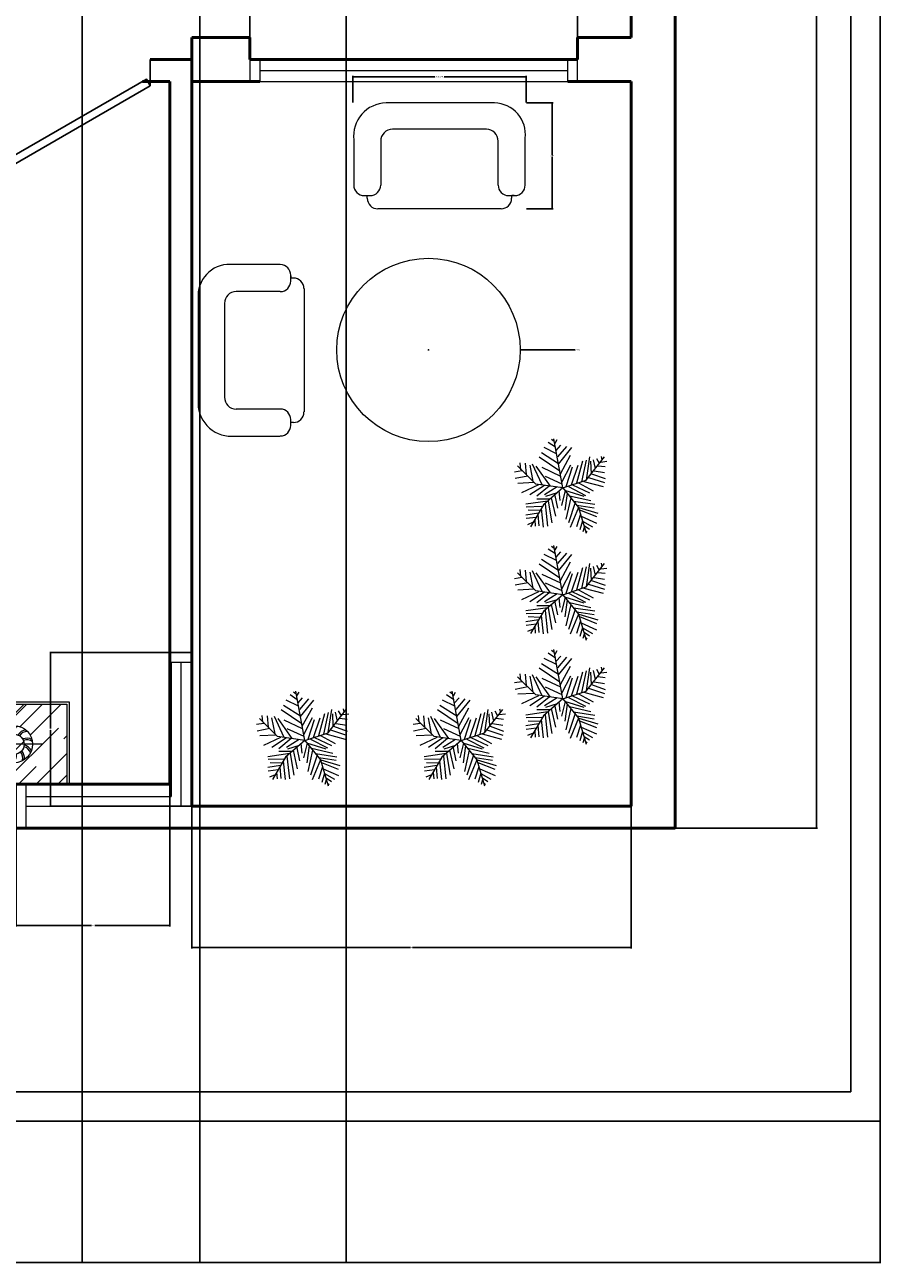
# Model space of a CAD drawing. Units: inches. Extents: x -28 to 483, y -584 to 51.
# Tile 3 of 6: x 270 to 445, y -584 to -330. Entities that reach past the tile are written whole.
import ezdxf

# ---------------------------------------------------------------- set-up
doc = ezdxf.new("R2010")
doc.units = ezdxf.units.IN
doc.header["$MEASUREMENT"] = 0
for name, color, linetype, lineweight in [('A-ANNO-DIMS', 2, 'Continuous', 18), ('A-DOOR', 4, 'Continuous', 25), ('A-FURN', 30, 'Continuous', 18), ('A-GLAZ', 5, 'Continuous', 18), ('A-WALL', 7, 'Continuous', 50), ('C-PROP', 7, 'Continuous', 25), ('tree', 3, 'Continuous', 13)]:
    doc.layers.add(name, color=color, linetype=linetype, lineweight=lineweight)
doc.styles.get("Standard").update_dxf_attribs({"font": 'arial.ttf'})
doc.dimstyles.get("Standard").update_dxf_attribs({"dimtxt": 0.18, "dimasz": 0.18, "dimexe": 0.18, "dimexo": 0.0625, "dimgap": 0.09, "dimtad": 0, "dimtih": 1, "dimtoh": 1, "dimdec": 4, "dimzin": 0, "dimdsep": 46, "dimtxsty": 'Standard', "dimcen": 0.09, "dimadec": 0, "dimazin": 0, "dimtfac": 1, "dimtdec": 4, "dimtofl": 0, "dimtmove": 0, "dimatfit": 3, "dimfxl": 1, "dimtolj": 1, "dimtzin": 0, "dimarcsym": 0})

# ---------------------------------------------------------------- blocks, each defined once
blk = doc.blocks.new('*U2')
for p, q in [((0, 0), (0, -6)), ((40, 0), (40, -6))]:
    blk.add_line(p, q)
blk.add_lwpolyline([(0, 0), (34.64, 20), (35.52, 18.48), (0.87, -1.52)], close=True)
blk.add_arc((0, 0), 40, 0, 30)
blk = doc.blocks.new('A$C64B41DC1')
for p, q in [((0, 2.5079), (2.9903, 2.5079)), ((0, 2.0879), (0, 2.5079)), ((0.012, 2.4618), (0.0581, 2.5079)), ((0.012, 2.3515), (0.1684, 2.5079)), ((0.012, 2.0999), (0.012, 2.5079)), ((0.0543, 2.2213), (0.3409, 2.5079)), ((0.1689, 2.4179), (0.2589, 2.5079)), ((0.3265, 2.386), (0.4484, 2.5079)), ((0.3699, 2.3332), (0.5445, 2.5079)), ((0.548, 2.5079), (0.548, 2.0999)), ((0.56, 2.5079), (0.56, 2.0879)), ((0.6301, 2.5079), (0.6301, 0.4779)), ((0.6401, 2.461), (0.6401, 2.5079)), ((0.6401, 2.5079), (2.344, 2.5079)), ((2.344, 2.5079), (2.3601, 2.5079)), ((2.344, 2.5079), (2.344, 2.461)), ((2.3601, 2.5079), (2.3601, 2.4761)), ((2.3601, 0.4779), (2.3601, 2.5079)), ((2.4303, 2.5079), (2.4303, 2.0879)), ((2.4423, 2.5079), (2.4423, 2.0999)), ((2.4423, 2.3333), (2.6169, 2.5079)), ((2.4423, 2.2145), (2.7357, 2.5079)), ((2.4423, 2.404), (2.5354, 2.4971)), ((2.705, 2.398), (2.8149, 2.5079)), ((2.7691, 2.3772), (2.8998, 2.5079)), ((2.7819, 2.3646), (2.9252, 2.5079)), ((2.9783, 2.0999), (2.9783, 2.5079)), ((2.9903, 2.0879), (2.9903, 2.5079)), ((0.2157, 2.0999), (0.548, 2.4322)), ((0.2299, 2.0999), (0.548, 2.418)), ((0.2804, 2.1597), (0.2804, 2.4481)), ((2.344, 2.461), (0.6401, 2.461)), ((0.6601, 2.4461), (1.4951, 2.4461)), ((0.6601, 2.4461), (0.6601, 0.5579)), ((1.4951, 2.4461), (0.6697, 2.4461)), ((2.3301, 2.4461), (1.4951, 2.4461)), ((2.3301, 0.5579), (2.3301, 2.4461)), ((2.7099, 2.1597), (2.7099, 2.4481)), ((0.2311, 2.2906), (0.2937, 2.3532)), ((2.6674, 2.2756), (2.7382, 2.3464)), ((2.7914, 2.1846), (2.9783, 2.3715)), ((0.012, 2.261), (0.0275, 2.2765)), ((0.1362, 2.3039), (0.4246, 2.3039)), ((0.2905, 2.2539), (0.3304, 2.2938)), ((0.3405, 2.3039), (0.3605, 2.3238)), ((2.8541, 2.3039), (2.5657, 2.3039)), ((2.5849, 2.2779), (2.6158, 2.3088)), ((2.6158, 2.3088), (2.6313, 2.3243)), ((2.7249, 2.3076), (2.7512, 2.3339)), ((2.7746, 2.0999), (2.9783, 2.3036)), ((2.9144, 2.2312), (2.9783, 2.2951)), ((0.0404, 2.0999), (0.1982, 2.2578)), ((0.1365, 2.0999), (0.251, 2.2144)), ((0.4194, 2.0999), (0.548, 2.2285)), ((2.4423, 2.1353), (2.5382, 2.2312)), ((2.4918, 2.0999), (2.6366, 2.2447)), ((0.4986, 2.0999), (0.548, 2.1493)), ((2.7831, 2.0999), (2.8678, 2.1846)), ((2.8962, 2.0999), (2.9783, 2.182)), ((0.56, 2.0879), (0, 2.0879)), ((0.548, 2.0999), (0.012, 2.0999)), ((0.5127, 2.0999), (0.548, 2.1352)), ((2.4303, 2.0879), (2.9903, 2.0879)), ((2.4423, 2.0999), (2.9783, 2.0999)), ((2.5172, 2.0999), (2.5269, 2.1096)), ((0.9415, 1.9902), (0.9415, 1.3975)), ((0.9715, 1.9906), (0.9715, 1.4076)), ((1.0015, 1.991), (1.0015, 1.4177)), ((1.0315, 1.9916), (1.0315, 1.4279)), ((2.3349, 1.8678), (0.6613, 1.3029)), ((0.8956, 1.1191), (2.3349, 1.8678)), ((1.6636, 1.6412), (0.6601, 1.6412)), ((1.5748, 1.6112), (0.6601, 1.6112)), ((2.3665, 1.295), (2.3665, 1.3839)), ((2.377, 1.295), (2.3822, 1.3891)), ((2.4032, 1.295), (2.4032, 1.3839)), ((2.4346, 1.295), (2.4346, 1.3839)), ((2.4451, 1.295), (2.4503, 1.3891)), ((2.4774, 1.2957), (2.4774, 1.3837)), ((2.5, 1.295), (2.5, 1.3839)), ((2.5105, 1.295), (2.5157, 1.3891)), ((2.5367, 1.295), (2.5367, 1.3839)), ((2.5471, 1.295), (2.5524, 1.3891)), ((2.5681, 1.295), (2.5681, 1.3839)), ((2.5918, 1.295), (2.5918, 1.3839)), ((2.6346, 1.2957), (2.6346, 1.3837)), ((2.6362, 1.2957), (2.6467, 1.3839)), ((2.6729, 1.295), (2.6624, 1.3839)), ((2.6938, 1.295), (2.6938, 1.3839)), ((2.7043, 1.295), (2.7095, 1.3891)), ((2.7127, 1.2957), (2.7232, 1.3839)), ((2.7253, 1.295), (2.7253, 1.3839)), ((2.7494, 1.295), (2.7389, 1.3839)), ((2.7718, 1.295), (2.7718, 1.3839)), ((2.7959, 1.295), (2.7854, 1.3839)), ((2.8146, 1.2957), (2.8146, 1.3837)), ((2.8146, 1.2957), (2.8146, 1.3837)), ((2.8282, 1.295), (2.8282, 1.3839)), ((2.8282, 1.295), (2.8282, 1.3839)), ((2.8523, 1.295), (2.8418, 1.3839)), ((2.8523, 1.295), (2.8418, 1.3839)), ((2.8653, 1.2966), (2.8688, 1.3861)), ((2.8711, 1.2957), (2.8711, 1.3837)), ((2.8711, 1.2957), (2.8875, 1.3822)), ((2.8713, 1.2927), (2.954, 1.3315)), ((2.8765, 1.2958), (2.9132, 1.3758)), ((2.8893, 1.3011), (2.9394, 1.3636)), ((2.3601, 1.2873), (2.8639, 1.2873)), ((2.8639, 1.2873), (2.8639, 0.1018)), ((2.8716, 1.2565), (2.9605, 1.2669)), ((2.8717, 1.2884), (2.9588, 1.3058)), ((2.8744, 1.2817), (2.9603, 1.2869)), ((2.3601, 1.2233), (2.7999, 1.2233)), ((2.7999, 1.2233), (2.7999, 0.1658)), ((2.8716, 1.2212), (2.9605, 1.2212)), ((2.8716, 1.1947), (2.9605, 1.2052)), ((2.8723, 1.2489), (2.9603, 1.2489)), ((2.3601, 1.1913), (2.7679, 1.1912)), ((2.7679, 1.1912), (2.7679, 0.1978)), ((2.8716, 1.181), (2.9605, 1.1705)), ((2.8716, 1.1595), (2.9605, 1.1595)), ((2.8716, 1.133), (2.9605, 1.1435)), ((2.8723, 1.1872), (2.9603, 1.1872)), ((2.8716, 1.1193), (2.9605, 1.1088)), ((2.8716, 1.1035), (2.9605, 1.093)), ((2.8716, 1.0965), (2.9605, 1.0965)), ((2.8716, 1.086), (2.9657, 1.0913)), ((2.8716, 1.0756), (2.9605, 1.0756)), ((2.8723, 1.1255), (2.9603, 1.1255)), ((2.8723, 1.0858), (2.9605, 1.0753)), ((2.8716, 1.0491), (2.9605, 1.0596)), ((2.8716, 1.0354), (2.9605, 1.0249)), ((2.8723, 1.0416), (2.9603, 1.0416)), ((2.8723, 0.9987), (2.9605, 1.0092)), ((2.8723, 0.985), (2.9605, 0.9745)), ((2.8723, 0.9735), (2.9603, 0.9735)), ((2.8716, 0.9346), (2.9605, 0.9241)), ((2.8723, 0.9408), (2.9603, 0.9408)), ((2.8723, 0.8979), (2.9605, 0.9084)), ((2.8723, 0.8726), (2.9603, 0.8726)), ((2.8723, 0.8505), (2.9603, 0.8505)), ((2.8716, 0.7885), (2.9605, 0.799)), ((2.8716, 0.7818), (2.9657, 0.787)), ((2.8716, 0.7503), (2.9657, 0.7556)), ((2.8716, 0.7204), (2.9605, 0.7309)), ((2.8716, 0.6995), (2.9605, 0.6995)), ((2.8723, 0.7571), (2.9605, 0.7466)), ((2.8716, 0.689), (2.9657, 0.6838)), ((2.8716, 0.6576), (2.9657, 0.6523)), ((2.8716, 0.6471), (2.9605, 0.6471)), ((2.8716, 0.5903), (2.9605, 0.6007)), ((0.7101, 0.5079), (2.2801, 0.5079)), ((2.882, 0.5582), (2.9657, 0.5536)), ((2.8909, 0.5263), (2.9657, 0.5222)), ((2.8928, 0.5169), (2.9605, 0.5169)), ((0.6301, 0.4779), (2.3601, 0.4779)), ((1.2465, 0.4625), (1.1576, 0.452)), ((1.2542, 0.1018), (1.2542, 0.4779)), ((1.3182, 0.1658), (1.3182, 0.4779)), ((1.3502, 0.1978), (1.3502, 0.4779)), ((2.8716, 0.4877), (2.9603, 0.4877)), ((2.8716, 0.4625), (2.9605, 0.452)), ((1.2465, 0.3746), (1.1576, 0.3851)), ((1.2465, 0.4365), (1.1577, 0.4365)), ((2.8716, 0.4365), (2.9603, 0.4365)), ((2.8716, 0.3746), (2.9605, 0.3851)), ((1.2465, 0.3684), (1.1577, 0.3684)), ((1.2285, 0.3357), (1.1577, 0.3357)), ((2.8716, 0.3684), (2.9603, 0.3684)), ((2.8896, 0.3357), (2.9603, 0.3357)), ((1.2355, 0.3092), (1.1576, 0.3)), ((1.2457, 0.2676), (1.1577, 0.2676)), ((2.8723, 0.2676), (2.9603, 0.2676)), ((2.8826, 0.3092), (2.9605, 0.3)), ((1.2457, 0.2423), (1.1576, 0.2319)), ((1.2465, 0.2057), (1.1576, 0.2161)), ((2.7679, 0.1978), (1.3502, 0.1978)), ((2.8716, 0.2057), (2.9605, 0.2161)), ((2.8723, 0.2423), (2.9605, 0.2319)), ((1.2465, 0.1742), (1.1524, 0.169)), ((1.2465, 0.1428), (1.1524, 0.1376)), ((1.2465, 0.1334), (1.1524, 0.1281)), ((1.2465, 0.1847), (1.1576, 0.1847)), ((1.2465, 0.1323), (1.1576, 0.1323)), ((1.2465, 0.1323), (1.1576, 0.1323)), ((2.7999, 0.1658), (1.3182, 0.1658)), ((2.8716, 0.1847), (2.9605, 0.1847)), ((2.8716, 0.1742), (2.9657, 0.169)), ((2.8716, 0.1428), (2.9657, 0.1376)), ((2.8716, 0.1334), (2.9657, 0.1281)), ((2.8716, 0.1323), (2.9605, 0.1323)), ((1.2465, 0.1), (1.1576, 0.1105)), ((1.2465, 0.1229), (1.1588, 0.1168)), ((1.2464, 0.1007), (1.1592, 0.0833)), ((1.2468, 0.0964), (1.1641, 0.0576)), ((1.2288, 0.088), (1.1787, 0.0255)), ((1.2415, 0.0933), (1.2049, 0.0133)), ((1.247, 0.0934), (1.2306, 0.0069)), ((1.2527, 0.0925), (1.2493, 0.003)), ((2.8639, 0.1018), (1.2542, 0.1018)), ((1.2658, 0.0941), (1.2762, 0.0052)), ((1.2899, 0.0941), (1.2899, 0.0052)), ((1.2999, 0.0941), (1.3051, 0)), ((1.3313, 0.0941), (1.3365, 0)), ((1.3523, 0.0941), (1.3575, 0)), ((1.3804, 0.0941), (1.3699, 0.0052)), ((1.4119, 0.0934), (1.4223, 0.0052)), ((1.4485, 0.0941), (1.438, 0.0052)), ((1.48, 0.0941), (1.4852, 0)), ((1.5114, 0.0941), (1.5166, 0)), ((1.5323, 0.0941), (1.5376, 0)), ((1.5638, 0.0941), (1.5638, 0.0105)), ((1.6021, 0.0941), (1.6021, 0.0052)), ((1.6336, 0.0941), (1.6336, 0.0052)), ((1.6702, 0.0941), (1.6702, 0.0052)), ((1.7017, 0.0941), (1.7017, 0.0052)), ((1.7122, 0.0941), (1.7174, 0)), ((1.7445, 0.0934), (1.7445, 0.0054)), ((1.7698, 0.0934), (1.7803, 0.0052)), ((1.8065, 0.0941), (1.796, 0.0052)), ((1.8274, 0.0941), (1.8274, 0.0052)), ((1.8379, 0.0941), (1.8431, 0)), ((1.8746, 0.0941), (1.8798, 0)), ((1.8955, 0.0941), (1.8955, 0.0052)), ((1.906, 0.0941), (1.9113, 0)), ((1.9384, 0.0934), (1.9384, 0.0054)), ((1.9609, 0.0941), (1.9609, 0.0052)), ((1.9636, 0.0934), (1.9741, 0.0052)), ((1.9714, 0.0941), (1.9766, 0)), ((1.9976, 0.0941), (1.9976, 0.0052)), ((2.0081, 0.0941), (2.0133, 0)), ((2.029, 0.0941), (2.029, 0.0052)), ((2.0395, 0.0941), (2.0447, 0)), ((2.0797, 0.0941), (2.0797, 0.0052)), ((2.0902, 0.0941), (2.0954, 0)), ((2.1216, 0.0941), (2.1269, 0)), ((2.1412, 0.0941), (2.1412, 0.0052)), ((2.1517, 0.0941), (2.1569, 0)), ((2.1831, 0.0941), (2.1884, 0)), ((2.2093, 0.0941), (2.2093, 0.0052)), ((2.2198, 0.0941), (2.225, 0)), ((2.2512, 0.0941), (2.2565, 0)), ((2.2603, 0.0934), (2.2707, 0.0052)), ((2.2969, 0.0941), (2.2864, 0.0052)), ((2.3089, 0.0934), (2.3193, 0.0052)), ((2.3455, 0.0941), (2.3351, 0.0052)), ((2.3665, 0.0941), (2.3665, 0.0052)), ((2.377, 0.0941), (2.3822, 0)), ((2.4032, 0.0941), (2.4032, 0.0052)), ((2.4346, 0.0941), (2.4346, 0.0052)), ((2.4451, 0.0941), (2.4503, 0)), ((2.4774, 0.0934), (2.4774, 0.0054)), ((2.5, 0.0941), (2.5, 0.0052)), ((2.5105, 0.0941), (2.5157, 0)), ((2.5367, 0.0941), (2.5367, 0.0052)), ((2.5471, 0.0941), (2.5524, 0)), ((2.5681, 0.0941), (2.5681, 0.0052)), ((2.5918, 0.0941), (2.5918, 0.0052)), ((2.6346, 0.0934), (2.6346, 0.0054)), ((2.6362, 0.0934), (2.6467, 0.0052)), ((2.6729, 0.0941), (2.6624, 0.0052)), ((2.6938, 0.0941), (2.6938, 0.0052)), ((2.7043, 0.0941), (2.7095, 0)), ((2.7127, 0.0934), (2.7232, 0.0052)), ((2.7253, 0.0941), (2.7253, 0.0052)), ((2.7494, 0.0941), (2.7389, 0.0052)), ((2.7718, 0.0941), (2.7718, 0.0052)), ((2.7959, 0.0941), (2.7854, 0.0052)), ((2.8146, 0.0934), (2.8146, 0.0054)), ((2.8282, 0.0941), (2.8282, 0.0052)), ((2.8523, 0.0941), (2.8418, 0.0052)), ((2.8653, 0.0925), (2.8688, 0.003)), ((2.8711, 0.0934), (2.8875, 0.0069)), ((2.8713, 0.0964), (2.954, 0.0576)), ((2.8716, 0.1229), (2.9593, 0.1168)), ((2.8717, 0.1007), (2.9588, 0.0833)), ((2.8744, 0.1074), (2.9603, 0.1022)), ((2.8765, 0.0933), (2.9132, 0.0133)), ((2.8893, 0.088), (2.9394, 0.0255))]:
    blk.add_line(p, q)
at = {"ltscale": 10}
for p, q in [((1.4859, 1.5812), (0.6601, 1.5812)), ((1.397, 1.5512), (0.6601, 1.5512))]:
    blk.add_line(p, q, dxfattribs=at)
for centre, radius in [((0.2804, 2.3039), 0.0942), ((0.2804, 2.3039), 0.051), ((2.7099, 2.3039), 0.0942), ((2.7099, 2.3039), 0.051)]:
    blk.add_circle(centre, radius)
for centre, radius, start, end in [((0.6601, 2.4761), 0.03, 180, 270), ((2.3301, 2.4761), 0.03, 270, 0), ((0.2417, 2.3614), 0.0462, 196.30017, 256.53802), ((0.2887, 2.3745), 0.0605, 172.17003, 218.48975), ((0.2828, 2.3731), 0.0462, 160.30017, 220.53802), ((0.3286, 2.3561), 0.0605, 136.17003, 182.48975), ((0.3231, 2.3585), 0.0462, 124.30017, 184.53802), ((0.3501, 2.3178), 0.0605, 100.17003, 146.48975), ((0.347, 2.323), 0.0462, 88.30017, 148.53802), ((1.0526, 2.3302), 0.3085, 175.30484, 198.69419), ((-0.8702, 2.0941), 1.6364, 4.80985, 9.18918), ((0.8579, 2.6278), 0.2948, 247.51785, 264.26696), ((0.728, 2.111), 0.245, 40.4189, 85.9871), ((1.0164, 5.7096), 3.3803, 266.81337, 276.16021), ((1.3963, 2.1044), 0.245, 94.0129, 139.5811), ((1.1858, 2.3288), 0.1943, 306.5711, 5.88998), ((1.5348, 2.2652), 0.1767, 151.77364, 201.69827), ((1.6986, 2.3355), 0.1943, 174.11002, 233.4289), ((1.1481, 2.2311), 0.3783, 353.49469, 19.18669), ((1.6871, 3.192), 0.8561, 257.74383, 273.62843), ((1.4882, 2.111), 0.245, 40.4189, 85.9871), ((1.8674, 1.9709), 0.3878, 68.20259, 108.9817), ((2.1269, 2.1044), 0.245, 94.0129, 139.5811), ((2.0342, 2.4856), 0.1563, 261.59582, 298.90918), ((1.9165, 2.3288), 0.1943, 333.73715, 5.88998), ((2.6058, 2.2028), 0.517, 163.60457, 172.3273), ((2.6433, 2.323), 0.0462, 31.46198, 91.69983), ((2.6402, 2.3178), 0.0605, 33.51025, 79.82997), ((2.6672, 2.3585), 0.0462, 355.46198, 55.69983), ((2.6617, 2.3561), 0.0605, 357.51025, 43.82997), ((2.7075, 2.3731), 0.0462, 319.46198, 19.69983), ((2.7016, 2.3745), 0.0605, 321.51025, 7.82997), ((2.7486, 2.3614), 0.0462, 283.46198, 343.69983), ((0.2153, 2.3276), 0.0462, 232.30017, 292.53802), ((0.2158, 2.3336), 0.0605, 244.17003, 290.48975), ((0.2457, 2.3659), 0.0605, 208.17003, 254.48975), ((0.3449, 2.2742), 0.0605, 64.17003, 110.48975), ((0.3455, 2.2802), 0.0462, 52.30017, 112.53802), ((0.3191, 2.2464), 0.0462, 16.30017, 76.53802), ((0.3151, 2.2419), 0.0605, 28.17003, 74.48975), ((2.6448, 2.2802), 0.0462, 67.46198, 127.69983), ((2.6454, 2.2742), 0.0605, 69.51025, 115.82997), ((2.6752, 2.2419), 0.0605, 105.51025, 151.82997), ((2.6712, 2.2464), 0.0462, 103.46198, 163.69983), ((2.7744, 2.3336), 0.0605, 249.51025, 295.82997), ((2.775, 2.3276), 0.0462, 247.46198, 307.69983), ((2.7446, 2.3659), 0.0605, 285.51025, 331.82997), ((0.2138, 2.2848), 0.0462, 268.30017, 328.53802), ((0.2107, 2.29), 0.0605, 280.17003, 326.48975), ((0.2377, 2.2493), 0.0462, 304.30017, 4.53802), ((0.2322, 2.2517), 0.0605, 316.17003, 2.48975), ((0.2779, 2.2347), 0.0462, 340.30017, 40.53802), ((0.272, 2.2333), 0.0605, 352.17003, 38.48975), ((0.7274, 2.2013), 0.0446, 314.4736, 42.17134), ((-1.6008, 2.277), 2.3618, 357.39054, 358.88764), ((1.9165, 2.3288), 0.1943, 320.94042, 333.73715), ((2.1347, 2.2313), 0.0459, 165.35061, 223.26844), ((2.7182, 2.2333), 0.0605, 141.51025, 187.82997), ((2.7123, 2.2347), 0.0462, 139.46198, 199.69983), ((2.7581, 2.2517), 0.0605, 177.51025, 223.82997), ((2.7526, 2.2493), 0.0462, 175.46198, 235.69983), ((2.7796, 2.29), 0.0605, 213.51025, 259.82997), ((2.7765, 2.2848), 0.0462, 211.46198, 271.69983), ((0.2688, 2.0945), 0.4956, 344.0243, 8.70709), ((1.204, 2.1778), 0.1681, 337.01697, 7.53676), ((1.5671, 2.1546), 0.0547, 142.08329, 220.902), ((1.9346, 2.1778), 0.1681, 337.01697, 7.53676), ((0.9385, 1.978), 0.1943, 126.5711, 185.88998), ((1.1858, 1.9714), 0.1943, 4.31813, 53.4289), ((1.5415, 2.0969), 0.1834, 175.22328, 196.23004), ((1.7059, 1.9714), 0.204, 127.11975, 175.09005), ((1.1965, 2.0983), 0.3299, 343.79543, 3.55541), ((1.9394, 1.991), 0.1651, 351.26213, 55.75721), ((2.4617, 2.0719), 0.3745, 173.82958, 196.4356), ((1.2687, 1.9248), 0.1223, 33.62799, 86.47438), ((1.7676, 1.0629), 0.9631, 69.65065, 105.96307), ((2.2748, 2.5795), 0.6373, 238.34989, 254.31375), ((0.7417, 2.0149), 0.057, 273.47085, 328.54118), ((0.728, 2.2025), 0.245, 274.0129, 278.34166), ((0.7246, 18.8439), 16.8552, 270.17399, 272.05214), ((1.3401, 1.9404), 0.0603, 49.09906, 101.37023), ((2.0911, 2.0123), 0.0478, 179.77267, 283.80184), ((1.0747, 1.2871), 0.1871, 14.1863, 69.12121), ((1.0274, 1.1334), 0.2527, 40.62904, 104.37123), ((0.7347, 1.1553), 0.1649, 347.31088, 116.44537), ((0.7101, 0.5579), 0.05, 180, 270), ((2.2801, 0.5579), 0.05, 270, 0)]:
    blk.add_arc(centre, radius, start, end)
for centre, major_axis, ratio, start_param, end_param in [((1.9938, 1.6262), (0, -0.7531), 0.68, 0.797284, 0.954936), ((2.0643, 1.466), (0, -0.5322), 0.68, 7.239912, 7.311536), ((1.9052, 1.7397), (0, -0.9842), 0.68, 0.74745, 0.979724), ((2.7455, 1.3081), (0, 0.3614), 0.68, 1.900046, 2.742661), ((2.7868, 1.3081), (0, 0.3614), 0.68, 1.900046, 2.614747), ((2.8372, 1.3081), (0, 0.3614), 0.68, 1.900046, 2.479658), ((2.8607, 1.3211), (0, 0.3614), 0.68, 1.938265, 2.479658), ((2.8057, 1.2079), (0, -0.1524), 0.68, 4.821745, 5.895886), ((2.4665, 0.8216), (0, -0.2664), 0.68, 2.006169, 3.565187), ((2.4513, 0.5069), (0, 0.502), 0.68, 5.095327, 6.553458), ((2.7862, 0.8069), (0, -0.2615), 0.68, 3.244645, 4.205018), ((2.396, 0.6032), (0, 0.3641), 0.68, -1.3172, 0.145284), ((2.7784, 0.8289), (0, -0.1802), 0.68, 3.227058, 4.318474), ((2.7821, 0.7971), (0, -0.1589), 0.68, 3.272942, 4.229533), ((2.3507, 0.5642), (0.0073, 0.3819), 0.56205, -1.21172, -0.009991), ((2.2964, 0.5771), (0, -0.3263), 0.68, 1.938944, 2.850232), ((2.0403, 1.6015), (0, -0.8763), 0.68, 6.849801, 6.887077), ((2.4005, 0.7132), (0, -0.1214), 0.68, 2.284368, 3.652258), ((2.3834, 0.7081), (0, 0.1147), 0.68, 4.593909, 6.585576), ((2.3774, 0.7653), (0, -0.0593), 0.68, 5.841311, 7.755362), ((2.3961, 0.7628), (0, -0.0317), 0.68, 1.462497, 5.046281), ((1.9938, 1.1295), (-0.0678, 0.7439), 0.610498, 3.917146, 4.063997), ((2.0643, 0.9693), (0, -0.5322), 0.68, 7.239912, 7.336618), ((1.9052, 1.243), (0, -0.9842), 0.68, 0.74745, 0.979724), ((2.7455, 0.8114), (-0.0599, 0.3735), 0.695517, 1.775813, 2.548612), ((2.7868, 0.8114), (0, 0.3614), 0.68, 1.900046, 2.614747), ((2.8607, 0.8243), (0, 0.3614), 0.68, 1.938265, 2.479658), ((2.4665, 0.3249), (0, -0.2664), 0.68, 2.006169, 3.565187), ((2.7862, 0.3102), (0, -0.2615), 0.68, 3.244645, 4.205018), ((2.4513, 0.0102), (0, 0.502), 0.68, 5.095327, 6.553458), ((2.7784, 0.3322), (0, -0.1802), 0.68, 3.227058, 4.318474), ((1.242, 0.9693), (0, -0.5322), 0.68, 6.586764, 6.677612), ((1.1714, 1.1295), (-0.1157, 0.7241), 0.59432, 3.291697, 3.50733), ((1.0828, 1.243), (0, -0.9842), 0.68, 0.565948, 0.680366), ((1.5283, 0.0674), (0, -0.3703), 0.68, 1.930561, 3.464283), ((1.5736, 0.1065), (0, 0.3641), 0.68, -1.3172, 0.476403), ((1.6289, 0.0102), (0, 0.502), 0.68, 6.655152, 6.661293), ((1.6289, 0.0102), (0, 0.502), 0.68, 5.095327, 5.911219), ((1.6442, 0.3249), (0, -0.2664), 0.68, 2.006169, 2.182797), ((1.9638, 0.3102), (0, -0.2615), 0.68, 4.015924, 4.205018), ((1.956, 0.3322), (0, -0.1802), 0.68, 3.770744, 4.318474), ((1.9597, 0.3004), (0, -0.1589), 0.68, 3.14258, 4.229533), ((2.0606, 0.5616), (0, -0.1803), 0.68, 5.194792, 5.929328), ((2.0606, 0.5616), (0, -0.1803), 0.68, 5.194792, 6.723255), ((2.1315, 0.6603), (0, -0.3155), 0.68, 5.328638, 6.949396), ((2.0549, 0.5656), (0, -0.1303), 0.68, 5.450951, 6.054641), ((2.0643, 0.9693), (0, -0.5322), 0.68, 6.20013, 6.677612), ((1.9938, 1.1295), (-0.0678, 0.7439), 0.610498, 3.199135, 3.592282), ((1.9052, 1.243), (0, -0.9842), 0.68, 0.565948, 0.680366), ((2.3507, 0.0674), (0, -0.3703), 0.68, 1.930561, 3.464283), ((2.396, 0.1065), (0, 0.3641), 0.68, -1.3172, 0.476403), ((2.4513, 0.0102), (0, 0.502), 0.68, 6.655152, 6.661293), ((2.7821, 0.3004), (0, -0.1589), 0.68, 3.272942, 4.229533), ((1.1933, 0.9181), (0, -0.624), 0.68, 0.378672, 0.625379), ((1.3091, 0.6603), (0, -0.3155), 0.68, 6.475719, 6.949396), ((1.1911, 1.1066), (0, 0.8458), 0.68, 3.421828, 3.728616), ((1.2179, 1.1047), (0, -0.8763), 0.68, 6.507006, 6.887077), ((1.474, 0.0804), (0, -0.3263), 0.68, 1.938944, 3.339184), ((2.0157, 0.9181), (0, -0.624), 0.68, -0.280078, 0.625379), ((2.0135, 1.1066), (0, 0.8458), 0.68, 2.978727, 3.728616), ((2.0403, 1.1047), (0, -0.8763), 0.68, 6.099302, 6.887077), ((2.2964, 0.0804), (0, -0.3263), 0.68, 1.938944, 3.339184), ((1.555, 0.2685), (0, -0.0593), 0.68, 3.732151, 7.755362), ((1.5781, 0.2165), (0, -0.1214), 0.68, 2.284368, 3.726131), ((1.561, 0.2114), (0, 0.1147), 0.68, 4.593909, 6.647252), ((2.3774, 0.2685), (0, -0.0593), 0.68, 3.732151, 7.755362), ((2.4005, 0.2165), (0, -0.1214), 0.68, 2.284368, 3.726131), ((2.3834, 0.2114), (0, 0.1147), 0.68, 4.593909, 6.647252), ((1.5737, 0.2661), (0, -0.0317), 0.68, 1.462497, 5.046281), ((2.3961, 0.2661), (0, -0.0317), 0.68, 1.462497, 5.046281)]:
    blk.add_ellipse(centre, major_axis=major_axis, ratio=ratio, start_param=start_param, end_param=end_param)
blk = doc.blocks.new('Trees - Imperial')
for p, q in [((-7.288, 39.707), (-21.778, 46.673)), ((-8.737, 47.138), (-17.069, 52.711)), ((-10.186, 53.64), (-13.084, 55.962)), ((0, 0), (-10.5, 57)), ((-9.099, 51.782), (-6.563, 55.962)), ((-7.65, 43.423), (-2.578, 49.46)), ((-5.839, 35.992), (4.667, 48.067)), ((-5.114, 27.632), (10.463, 46.673)), ((-48.585, 21.131), (-49.309, 29.026)), ((-3.665, 19.273), (-27.574, 35.527)), ((-5.114, 28.097), (-24.676, 40.636)), ((-2.941, 16.486), (8.652, 37.85)), ((16.259, 5.805), (23.142, 31.348)), ((22.055, 7.198), (27.489, 32.277)), ((27, 9), (48, 36)), ((27.127, 9.056), (31.112, 35.992)), ((31.836, 30.883), (32.561, 16.486)), ((35.096, 32.741), (37.27, 22.524)), ((38.719, 34.134), (41.979, 28.561)), ((43.791, 29.954), (51.036, 30.883)), ((44.153, 36.456), (45.239, 32.741)), ((-47.498, 19.737), (-55.83, 18.344)), ((-31.5, 4.5), (-52.5, 25.5)), ((-43.513, 28.561), (-42.427, 15.558)), ((-38.442, 26.239), (-34.819, 7.663)), ((-35.544, 28.097), (-24.314, 3.947)), ((-14.533, 2.09), (-30.834, 25.31)), ((-24.314, 23.917), (-2.941, 13.7)), ((-1.129, 6.734), (9.014, 26.704)), ((3.942, 1.625), (11.187, 24.381)), ((10.101, 3.483), (17.708, 26.239)), ((33.285, 16.486), (48.862, 10.913)), ((36.183, 19.737), (48.137, 17.88)), ((40.53, 25.775), (48.862, 24.846)), ((-40.615, 13.7), (-55.105, 10.913)), ((-33.37, 6.269), (-52.207, 5.34)), ((-28.299, 3.483), (-47.86, -5.805)), ((-21.416, 3.018), (-38.079, -8.128)), ((0, 0), (-31.5, 4.5)), ((-15.982, 2.09), (-30.11, -9.521)), ((0, 0), (-22.5, -19.5)), ((-6.563, 1.161), (-21.416, -8.128)), ((-20.691, 13.7), (-1.129, 4.876)), ((0, 0), (27, 9)), ((0, 0), (18, -22.5)), ((6.478, 1.625), (26.04, -8.592)), ((11.187, 3.483), (30.749, -5.805)), ((18.07, 5.805), (35.096, -3.483)), ((24.229, 7.663), (46.688, 1.625)), ((29.662, 12.307), (48.137, 6.269)), ((-15.257, -12.772), (-30.11, -12.772)), ((-6.563, -5.805), (-19.967, -9.985)), ((-13.446, -11.378), (-8.737, -32.741)), ((-9.461, -8.592), (-6.201, -23.453)), ((-4.752, -3.483), (-3.665, -14.629)), ((2.493, -3.019), (-1.491, -20.202)), ((1.769, -2.555), (24.229, -9.521)), ((5.029, -6.27), (2.131, -25.775)), ((9.014, -11.378), (3.58, -35.992)), ((7.565, -9.056), (32.198, -14.629)), ((-17.431, -15.094), (-42.789, -18.809)), ((-24.314, -21.596), (-42.427, -22.06)), ((-26.849, -26.24), (-40.253, -25.775)), ((-22.5, -19.5), (-37.5, -45)), ((-25.038, -23.918), (-22.865, -45.281)), ((-20.691, -18.345), (-17.793, -44.352)), ((-17.069, -15.094), (-12.721, -40.172)), ((14.085, -16.951), (6.478, -40.172)), ((18.07, -22.524), (8.289, -45.745)), ((12.274, -15.094), (36.907, -18.809)), ((16.259, -19.738), (36.183, -22.989)), ((18, -22.5), (27, -52.5)), ((18.433, -22.524), (40.53, -29.026)), ((19.157, -25.311), (38.719, -33.206)), ((-28.299, -29.026), (-42.789, -31.348)), ((-30.834, -34.135), (-42.427, -35.528)), ((-34.457, -39.708), (-40.978, -42.494)), ((-32.646, -36.921), (-31.921, -44.352)), ((-29.023, -30.884), (-27.936, -43.887)), ((20.244, -30.419), (15.897, -44.816)), ((22.78, -37.85), (19.519, -48.532)), ((21.331, -32.741), (39.081, -40.636)), ((22.78, -38.314), (34.372, -44.816)), ((24.591, -45.745), (23.142, -50.854)), ((24.591, -43.423), (30.749, -47.603)), ((26.764, -49.925), (28.213, -50.854))]:
    blk.add_line(p, q)
blk = doc.blocks.new('CHAIR-ARM')
for p, q in [((16.78, 35.16), (7.22, 35.16)), ((19, 31.79), (19, 33)), ((19, 32.88), (19, 32.4)), ((19.54, 32.4), (19, 32.4)), ((0, 28.91), (0, 6.66)), ((16.84, 29.63), (7.82, 29.63)), ((21.71, 30.23), (21.71, 4.97)), ((5.41, 27.22), (5.41, 7.98)), ((7.82, 5.58), (16.84, 5.58)), ((19, 2.21), (19, 3.41)), ((19.54, 2.81), (19, 2.81)), ((7.58, 0.04), (16.78, 0.04))]:
    blk.add_line(p, q)
for centre, radius, start, end in [((6.45, 28.76), 6.45, 83.159, 178.6697), ((16.84, 33), 2.16, 0, 90), ((16.84, 31.79), 2.16, 270, 0), ((19.54, 30.23), 2.16, 0, 90), ((7.82, 27.22), 2.41, 90, 180), ((7.82, 7.98), 2.41, 180, 270), ((6.81, 6.81), 6.81, 181.2564, 276.501), ((16.84, 3.41), 2.16, 0, 90), ((19.54, 4.97), 2.16, 270, 0), ((16.84, 2.21), 2.16, 270, 0)]:
    blk.add_arc(centre, radius, start, end)
blk = doc.blocks.new('*D17')
at = {"layer": 'A-ANNO-DIMS', "color": 0, "lineweight": -2, "transparency": 16777216}
for p, q in [((336.77, -345.94), (336.77, -340.49)), ((336.95, -340.67), (353.6, -340.67)), ((372.14, -340.67), (355.5, -340.67)), ((372.32, -345.94), (372.32, -340.49))]:
    blk.add_line(p, q, dxfattribs=at)
at = {"layer": 'A-ANNO-DIMS', "color": 0, "transparency": 16777216}
for points in [[(336.95, -340.64), (336.95, -340.7), (336.77, -340.67)], [(372.14, -340.64), (372.14, -340.7), (372.32, -340.67)]]:
    blk.add_solid(points, dxfattribs=at)
at = {"layer": 'Defpoints', "color": 0, "transparency": 16777216}
for p in [(372.32, -340.67), (336.77, -346), (372.32, -346)]:
    blk.add_point(p, dxfattribs=at)
at = {"layer": 'A-ANNO-DIMS', "color": 0, "transparency": 16777216, "insert": (354.55, -340.67), "char_height": 0.18, "attachment_point": 5}
blk.add_mtext('\\A1;CHAIR 36 TYP.', dxfattribs=at)
blk = doc.blocks.new('*D18')
at = {"layer": 'A-ANNO-DIMS', "color": 0, "lineweight": -2, "transparency": 16777216}
for p, q in [((372.39, -346), (377.84, -346)), ((377.66, -346.18), (377.66, -356.68)), ((377.66, -367.53), (377.66, -357.04)), ((372.39, -367.71), (377.84, -367.71))]:
    blk.add_line(p, q, dxfattribs=at)
at = {"layer": 'A-ANNO-DIMS', "color": 0, "transparency": 16777216}
for points in [[(377.63, -346.18), (377.69, -346.18), (377.66, -346)], [(377.63, -367.53), (377.69, -367.53), (377.66, -367.71)]]:
    blk.add_solid(points, dxfattribs=at)
at = {"layer": 'Defpoints', "color": 0, "transparency": 16777216}
for p in [(372.32, -346), (372.32, -367.71), (377.66, -367.71)]:
    blk.add_point(p, dxfattribs=at)
at = {"layer": 'A-ANNO-DIMS', "color": 0, "transparency": 16777216, "insert": (377.66, -356.86), "char_height": 0.18, "attachment_point": 5}
blk.add_mtext('\\A1;22 TYP.', dxfattribs=at)
blk = doc.blocks.new('*D19')
at = {"layer": 'A-ANNO-DIMS', "color": 0, "lineweight": -2, "transparency": 16777216}
for p, q in [((12.84, -554.65), (12.84, -583.72)), ((444.84, -554.65), (444.84, -583.72)), ((13.02, -583.54), (228.55, -583.54)), ((444.66, -583.54), (229.13, -583.54))]:
    blk.add_line(p, q, dxfattribs=at)
at = {"layer": 'A-ANNO-DIMS', "color": 0, "transparency": 16777216}
for points in [[(13.02, -583.51), (13.02, -583.57), (12.84, -583.54)], [(444.66, -583.51), (444.66, -583.57), (444.84, -583.54)]]:
    blk.add_solid(points, dxfattribs=at)
at = {"layer": 'Defpoints', "color": 0, "transparency": 16777216}
for p in [(12.84, -554.59), (444.84, -554.59), (444.84, -583.54)]:
    blk.add_point(p, dxfattribs=at)
at = {"layer": 'A-ANNO-DIMS', "color": 0, "transparency": 16777216, "insert": (228.84, -583.54), "char_height": 0.18, "attachment_point": 5}
blk.add_mtext('\\A1;432', dxfattribs=at)
blk = doc.blocks.new('*D22')
at = {"layer": 'A-ANNO-DIMS', "color": 0, "lineweight": -2, "transparency": 16777216}
for p, q in [((402.905662, -17.587684), (431.973162, -17.587684)), ((431.793162, -17.767684), (431.793162, -255.907684)), ((431.793162, -494.407684), (431.793162, -256.267684)), ((402.905662, -494.587684), (431.973162, -494.587684))]:
    blk.add_line(p, q, dxfattribs=at)
at = {"layer": 'A-ANNO-DIMS', "color": 0, "transparency": 16777216}
for points in [[(431.763162, -17.767684), (431.823162, -17.767684), (431.793162, -17.587684)], [(431.763162, -494.407684), (431.823162, -494.407684), (431.793162, -494.587684)]]:
    blk.add_solid(points, dxfattribs=at)
at = {"layer": 'Defpoints', "color": 0, "transparency": 16777216}
for p in [(402.843162, -17.587684), (402.843162, -494.587684), (431.793162, -494.587684)]:
    blk.add_point(p, dxfattribs=at)
at = {"layer": 'A-ANNO-DIMS', "color": 0, "transparency": 16777216, "insert": (431.793162, -256.087684), "char_height": 0.18, "attachment_point": 5}
blk.add_mtext('\\A1;477', dxfattribs=at)
blk = doc.blocks.new('*D30')
at = {"layer": 'A-ANNO-DIMS', "color": 0, "lineweight": -2, "transparency": 16777216}
for p, q in [((305.44, -116.65), (305.44, -583.72)), ((335.44, -116.65), (335.44, -583.72)), ((305.62, -583.54), (320.22, -583.54)), ((335.26, -583.54), (320.66, -583.54))]:
    blk.add_line(p, q, dxfattribs=at)
at = {"layer": 'A-ANNO-DIMS', "color": 0, "transparency": 16777216}
for points in [[(305.62, -583.51), (305.62, -583.57), (305.44, -583.54)], [(335.26, -583.51), (335.26, -583.57), (335.44, -583.54)]]:
    blk.add_solid(points, dxfattribs=at)
at = {"layer": 'Defpoints', "color": 0, "transparency": 16777216}
for p in [(305.44, -116.59), (335.44, -116.59), (335.44, -583.54)]:
    blk.add_point(p, dxfattribs=at)
at = {"layer": 'A-ANNO-DIMS', "color": 0, "transparency": 16777216, "insert": (320.44, -583.54), "char_height": 0.18, "attachment_point": 5}
blk.add_mtext('\\A1;30', dxfattribs=at)
blk = doc.blocks.new('*D31')
at = {"layer": 'A-ANNO-DIMS', "color": 0, "lineweight": -2, "transparency": 16777216}
for p, q in [((281.34, -116.65), (281.34, -583.72)), ((305.44, -116.65), (305.44, -583.72)), ((281.52, -583.54), (293.08, -583.54)), ((305.26, -583.54), (293.7, -583.54))]:
    blk.add_line(p, q, dxfattribs=at)
at = {"layer": 'A-ANNO-DIMS', "color": 0, "transparency": 16777216}
for points in [[(281.52, -583.51), (281.52, -583.57), (281.34, -583.54)], [(305.26, -583.51), (305.26, -583.57), (305.44, -583.54)]]:
    blk.add_solid(points, dxfattribs=at)
at = {"layer": 'Defpoints', "color": 0, "transparency": 16777216}
for p in [(281.34, -116.59), (305.44, -116.59), (305.44, -583.54)]:
    blk.add_point(p, dxfattribs=at)
at = {"layer": 'A-ANNO-DIMS', "color": 0, "transparency": 16777216, "insert": (293.39, -583.54), "char_height": 0.18, "attachment_point": 5}
blk.add_mtext('\\A1;24.1', dxfattribs=at)
blk = doc.blocks.new('*D32')
at = {"layer": 'A-ANNO-DIMS', "color": 0, "lineweight": -2, "transparency": 16777216}
for p, q in [((303.84, -490.15), (303.84, -519.22)), ((393.84, -490.15), (393.84, -519.22)), ((304.02, -519.04), (348.62, -519.04)), ((393.66, -519.04), (349.06, -519.04))]:
    blk.add_line(p, q, dxfattribs=at)
at = {"layer": 'A-ANNO-DIMS', "color": 0, "transparency": 16777216}
for points in [[(304.02, -519.01), (304.02, -519.07), (303.84, -519.04)], [(393.66, -519.01), (393.66, -519.07), (393.84, -519.04)]]:
    blk.add_solid(points, dxfattribs=at)
at = {"layer": 'Defpoints', "color": 0, "transparency": 16777216}
for p in [(303.84, -490.09), (393.84, -490.09), (303.84, -519.04)]:
    blk.add_point(p, dxfattribs=at)
at = {"layer": 'A-ANNO-DIMS', "color": 0, "transparency": 16777216, "insert": (348.84, -519.04), "char_height": 0.18, "attachment_point": 5}
blk.add_mtext('\\A1;90', dxfattribs=at)
blk = doc.blocks.new('*D41')
at = {"layer": 'A-ANNO-DIMS', "color": 0, "lineweight": -2, "transparency": 16777216}
for p, q in [((315.72, -337.03), (315.72, 50.54)), ((315.9, 50.36), (348.97, 50.36)), ((382.64, 50.36), (349.58, 50.36)), ((382.82, -337.03), (382.82, 50.54))]:
    blk.add_line(p, q, dxfattribs=at)
at = {"layer": 'A-ANNO-DIMS', "color": 0, "transparency": 16777216}
for points in [[(315.9, 50.39), (315.9, 50.33), (315.72, 50.36)], [(382.64, 50.39), (382.64, 50.33), (382.82, 50.36)]]:
    blk.add_solid(points, dxfattribs=at)
at = {"layer": 'Defpoints', "color": 0, "transparency": 16777216}
for p in [(382.82, 50.36), (315.72, -337.09), (382.82, -337.09)]:
    blk.add_point(p, dxfattribs=at)
at = {"layer": 'A-ANNO-DIMS', "color": 0, "transparency": 16777216, "insert": (349.27, 50.36), "char_height": 0.18, "attachment_point": 5}
blk.add_mtext('\\A1;67.1', dxfattribs=at)
blk = doc.blocks.new('*D43')
at = {"layer": 'A-ANNO-DIMS', "color": 0, "lineweight": -2, "transparency": 16777216}
for p, q in [((267.84, -485.65), (267.84, -514.72)), ((299.34, -485.65), (299.34, -514.72)), ((268.02, -514.54), (283.27, -514.54)), ((299.16, -514.54), (283.92, -514.54))]:
    blk.add_line(p, q, dxfattribs=at)
at = {"layer": 'A-ANNO-DIMS', "color": 0, "transparency": 16777216}
for points in [[(268.02, -514.51), (268.02, -514.57), (267.84, -514.54)], [(299.16, -514.51), (299.16, -514.57), (299.34, -514.54)]]:
    blk.add_solid(points, dxfattribs=at)
at = {"layer": 'Defpoints', "color": 0, "transparency": 16777216}
for p in [(267.84, -485.59), (299.34, -485.59), (267.84, -514.54)]:
    blk.add_point(p, dxfattribs=at)
at = {"layer": 'A-ANNO-DIMS', "color": 0, "transparency": 16777216, "insert": (283.59, -514.54), "char_height": 0.18, "attachment_point": 5}
blk.add_mtext('\\A1;31.5', dxfattribs=at)
blk = doc.blocks.new('*D44')
at = {"layer": 'A-ANNO-DIMS', "color": 0, "lineweight": -2, "transparency": 16777216}
for p, q in [((303.78, -458.59), (274.71, -458.59)), ((274.89, -458.77), (274.89, -474.16)), ((274.89, -489.91), (274.89, -474.52)), ((303.78, -490.09), (274.71, -490.09))]:
    blk.add_line(p, q, dxfattribs=at)
at = {"layer": 'A-ANNO-DIMS', "color": 0, "transparency": 16777216}
for points in [[(274.86, -458.77), (274.92, -458.77), (274.89, -458.59)], [(274.86, -489.91), (274.92, -489.91), (274.89, -490.09)]]:
    blk.add_solid(points, dxfattribs=at)
at = {"layer": 'Defpoints', "color": 0, "transparency": 16777216}
for p in [(274.89, -458.59), (303.84, -458.59), (303.84, -490.09)]:
    blk.add_point(p, dxfattribs=at)
at = {"layer": 'A-ANNO-DIMS', "color": 0, "transparency": 16777216, "insert": (274.89, -474.34), "char_height": 0.18, "attachment_point": 5}
blk.add_mtext('\\A1;31.5', dxfattribs=at)
blk = doc.blocks.new('*D49')
at = {"layer": 'A-ANNO-DIMS', "color": 0, "lineweight": -2, "transparency": 16777216}
for p, q in [((352.21, -396.61), (352.39, -396.61)), ((352.3, -396.7), (352.3, -396.52)), ((382.35, -396.61), (371.26, -396.61))]:
    blk.add_line(p, q, dxfattribs=at)
at = {"layer": 'A-ANNO-DIMS', "color": 0, "transparency": 16777216}
blk.add_solid([(371.26, -396.58), (371.26, -396.64), (371.08, -396.61)], dxfattribs=at)
at = {"layer": 'Defpoints', "color": 0, "transparency": 16777216}
for p in [(333.51, -396.61), (371.08, -396.61)]:
    blk.add_point(p, dxfattribs=at)
at = {"layer": 'A-ANNO-DIMS', "color": 0, "transparency": 16777216, "insert": (382.84, -396.61), "char_height": 0.18, "attachment_point": 5}
blk.add_mtext('\\A1;∅37.56', dxfattribs=at)

msp = doc.modelspace()

# ---------------------------------------------------------------- linework, layer by layer
at = {"layer": 'A-FURN'}
msp.add_circle((352.2963, -396.6097), 18.7817, dxfattribs=at)
at = {"layer": 'A-GLAZ'}
for p, q in [((315.7242, -337.0877), (315.7242, -341.5877)), ((382.8208, -337.0877), (315.7242, -337.0877)), ((317.7242, -337.0877), (317.7242, -341.5877)), ((380.8208, -341.5877), (380.8208, -337.0877)), ((382.8208, -341.5877), (382.8208, -337.0877)), ((317.7242, -339.3377), (380.8208, -339.3377)), ((315.7242, -341.5877), (382.8208, -341.5877)), ((299.3432, -458.5877), (303.8432, -458.5877)), ((299.3432, -460.5877), (303.8432, -460.5877)), ((299.5932, -460.5877), (299.5932, -488.0877)), ((301.5932, -460.5877), (301.5932, -490.0877)), ((269.8432, -485.5877), (269.8432, -494.5877)), ((269.8432, -488.0877), (299.5932, -488.0877)), ((269.8432, -490.0877), (301.5932, -490.0877))]:
    msp.add_line(p, q, dxfattribs=at)
at = {"layer": 'A-WALL'}
for p, q in [((402.8432, -17.5877), (402.8432, -494.5877)), ((393.8432, -193.0877), (393.8432, -332.5877)), ((303.8432, -332.5877), (315.7242, -332.5877)), ((303.8432, -332.5877), (303.8432, -341.5877)), ((315.7242, -332.5877), (315.7242, -337.0877)), ((382.8208, -332.5877), (382.8208, -337.0877)), ((382.8208, -332.5877), (393.8432, -332.5877)), ((295.2944, -337.0877), (303.8432, -337.0877)), ((315.7242, -337.0877), (382.8208, -337.0877)), ((293.7033, -341.5877), (299.3432, -341.5877)), ((299.3432, -341.5877), (299.3432, -485.5877)), ((303.8432, -341.5877), (303.8432, -490.0877)), ((303.8432, -341.5877), (317.7242, -341.5877)), ((380.8208, -341.5877), (393.8432, -341.5877)), ((393.8432, -341.5877), (393.8432, -490.0877)), ((299.3432, -485.5877), (60.8432, -485.5877)), ((303.8432, -490.0877), (393.8432, -490.0877)), ((402.8432, -494.5877), (51.8432, -494.5877))]:
    msp.add_line(p, q, dxfattribs=at)
at = {"layer": 'C-PROP'}
for p, q in [((444.8432, 21.4123), (444.8432, -554.5877)), ((438.8432, 15.4123), (438.8432, -548.5877)), ((438.8432, -548.5877), (18.8432, -548.5877)), ((444.8432, -554.5877), (12.8432, -554.5877))]:
    msp.add_line(p, q, dxfattribs=at)

# ---------------------------------------------------------------- block references
at = {"layer": 'A-DOOR', "xscale": 0.9, "yscale": 0.9, "zscale": 0.9, "rotation": 180}
msp.add_blockref('*U2', (295.2944, -342.4877), dxfattribs=at)
at = {"layer": 'A-FURN', "rotation": 269.9999999999999}
msp.add_blockref('CHAIR-ARM', (336.9458, -346.0044), dxfattribs=at)
at = {"layer": 'A-FURN'}
msp.add_blockref('CHAIR-ARM', (305.091, -414.289), dxfattribs=at)
at = {"layer": 'A-FURN', "xscale": 40.13733178260718, "yscale": 40.13733178260718, "zscale": 40.13733178260718, "rotation": 180}
msp.add_blockref('A$C64B41DC1', (278.681, -384.9271), dxfattribs=at)
at = {"layer": 'tree', "xscale": 0.1769942182073353, "yscale": 0.1769942182073353, "zscale": 0.1769942182073353}
for p in [(379.8362, -424.8921), (379.8362, -446.7569), (379.8362, -468.0883), (326.9758, -476.6209), (359.0124, -476.6209)]:
    msp.add_blockref('Trees - Imperial', p, dxfattribs=at)

# ---------------------------------------------------------------- dimensions: what is measured, and where the dimension line sits
at = {"layer": 'A-ANNO-DIMS'}
for base, p1, p2, override, picture, middle in [((382.8208, 50.3623), (315.7242, -337.0877), (382.8208, -337.0877), {"dimdec": 1, "dimlfac": 1, "dimrnd": 0, "dimzin": 0, "dimdsep": 46, "dimlunit": 2}, '*D41', (349.2725, 50.3623)), ((305.4421, -583.5377), (281.3432, -116.5877), (305.4421, -116.5877), {"dimdec": 1, "dimlfac": 1, "dimrnd": 0, "dimzin": 0, "dimdsep": 46, "dimlunit": 2}, '*D31', (293.3926, -583.5377)), ((335.4421, -583.5377), (305.4421, -116.5877), (335.4421, -116.5877), {"dimdec": 0, "dimlfac": 1, "dimrnd": 0, "dimzin": 0, "dimdsep": 46, "dimlunit": 2}, '*D30', (320.4421, -583.5377)), ((444.8432, -583.5377), (12.8432, -554.5877), (444.8432, -554.5877), {"dimdec": 0, "dimlfac": 1, "dimrnd": 0, "dimzin": 0, "dimdsep": 46, "dimlunit": 2}, '*D19', (228.8432, -583.5377))]:
    dim = msp.add_linear_dim(base=base, p1=p1, p2=p2, dimstyle='Standard', override=override, dxfattribs=at)
    dim.commit()
    dim.dimension.update_dxf_attribs({"geometry": picture, "text_midpoint": middle})
for base, p1, p2, angle, override, picture, middle in [((431.7932, -494.5877), (402.8432, -17.5877), (402.8432, -494.5877), 270, {"dimdec": 0, "dimlfac": 1, "dimrnd": 0, "dimzin": 0, "dimdsep": 46, "dimlunit": 2}, '*D22', (431.7932, -256.0877)), ((274.8932, -458.5877), (303.8432, -490.0877), (303.8432, -458.5877), 90, {"dimdec": 1, "dimlfac": 1, "dimrnd": 0, "dimzin": 0, "dimdsep": 46, "dimlunit": 2}, '*D44', (274.8932, -474.3377)), ((267.8432, -514.5377), (299.3432, -485.5877), (267.8432, -485.5877), 180, {"dimdec": 1, "dimlfac": 1, "dimrnd": 0, "dimzin": 0, "dimdsep": 46, "dimlunit": 2}, '*D43', (283.5932, -514.5377)), ((303.8432, -519.0377), (393.8432, -490.0877), (303.8432, -490.0877), 180, {"dimdec": 0, "dimlfac": 1, "dimrnd": 0, "dimzin": 0, "dimdsep": 46, "dimlunit": 2}, '*D32', (348.8432, -519.0377))]:
    dim = msp.add_linear_dim(base=base, p1=p1, p2=p2, angle=angle, dimstyle='Standard', override=override, dxfattribs=at)
    dim.commit()
    dim.dimension.update_dxf_attribs({"geometry": picture, "text_midpoint": middle})
dim = msp.add_linear_dim(base=(372.3236, -340.6719), p1=(336.773, -346.0044), p2=(372.3236, -346.0044), text='CHAIR <> TYP.', dimstyle='Standard', override={"dimdec": 0, "dimlfac": 1, "dimrnd": 0, "dimzin": 0, "dimdsep": 46, "dimlunit": 2}, dxfattribs=at)
dim.commit()
dim.dimension.update_dxf_attribs({"geometry": '*D17', "text_midpoint": (354.5483, -340.6719)})
dim = msp.add_linear_dim(base=(377.6562, -367.7125), p1=(372.3236, -346.0044), p2=(372.3236, -367.7125), angle=270, text='<> TYP.', dimstyle='Standard', override={"dimdec": 0, "dimlfac": 1, "dimrnd": 0, "dimzin": 0, "dimdsep": 46, "dimlunit": 2}, dxfattribs=at)
dim.commit()
dim.dimension.update_dxf_attribs({"geometry": '*D18', "text_midpoint": (377.6562, -356.8585)})
dim = msp.add_diameter_dim_2p(p1=(333.5146, -396.6093), p2=(371.0781, -396.61), dimstyle='Standard', override={"dimdec": 2, "dimlfac": 1, "dimrnd": 0, "dimzin": 0, "dimdsep": 46, "dimlunit": 2}, dxfattribs=at)
dim.commit()
dim.dimension.update_dxf_attribs({"geometry": '*D49', "text_midpoint": (382.3471, -396.6102), "dimtype": 163})

doc.saveas('drawing.dxf')
